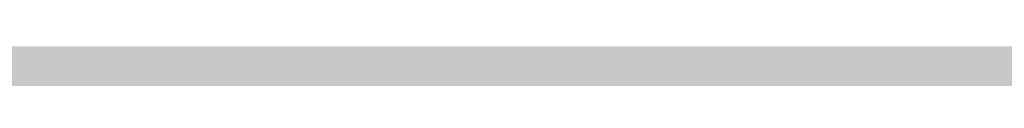
# Model space of a CAD drawing. Units: feet. Extents: x 3168 to 4724, y 827 to 1477.
# Tile 245 of 256: x 3383.8327 to 3384.3079, y 1099.0007 to 1099.0148. Entities that reach past the tile are written whole.
import ezdxf

# ---------------------------------------------------------------- set-up
doc = ezdxf.new("R2010")
doc.units = ezdxf.units.FT
doc.layers.add('A-ELEV', color=7, linetype='Continuous', lineweight=35)
doc.layers.add('A-ELEV-PATT', color=8, linetype='Continuous', lineweight=13)

msp = doc.modelspace()

# ---------------------------------------------------------------- hatches: boundary and pattern name
at = {"layer": 'A-ELEV-PATT'}
h = msp.add_hatch(color=256, dxfattribs=at)
h.dxf.hatch_style = 1
edge = h.paths.add_edge_path()
edge.add_ellipse((3552.90576, 979.22014), major_axis=(36.74492, 0), ratio=0.48484848, start_angle=0, end_angle=360)
edge = h.paths.add_edge_path()
edge.add_ellipse((3559.89164, 929.25228), major_axis=(36.74492, 0), ratio=0.48484848, start_angle=0, end_angle=360)
edge = h.paths.add_edge_path()
edge.add_line((3299.31681, 1198.60608), (3479.91671, 1198.60608))
edge.add_line((3479.91671, 1198.60608), (3479.91671, 1209.86857))
edge.add_spline(control_points=[(3479.91671, 1209.86857), (3464.30116, 1209.86857), (3448.6856, 1209.86857), (3410.94914, 1209.86857), (3388.82823, 1209.86857), (3355.64688, 1209.86857), (3344.58642, 1209.86857), (3327.99574, 1209.86857), (3322.46552, 1209.86857), (3314.17018, 1209.86857), (3311.40507, 1209.86857), (3307.2574, 1209.86857), (3305.87484, 1209.86857), (3303.801, 1209.86857), (3303.10973, 1209.86857), (3302.07281, 1209.86857), (3301.72717, 1209.86857), (3301.20871, 1209.86857), (3301.03589, 1209.86857), (3300.77666, 1209.86857), (3300.69025, 1209.86857), (3300.56064, 1209.86857), (3300.51743, 1209.86857), (3300.45263, 1209.86857), (3300.43102, 1209.86857), (3300.39862, 1209.86857), (3300.38782, 1209.86857), (3300.36622, 1209.86857), (3300.34568, 1209.86857), (3300.34555, 1209.86857), (3300.3455, 1209.86857), (3300.3433, 1209.86857), (3300.34115, 1209.86857), (3300.33791, 1209.86857), (3300.33683, 1209.86857), (3300.33394, 1209.86857), (3300.33213, 1209.86857), (3300.32552, 1209.86858), (3300.32071, 1209.86858), (3300.31092, 1209.86859), (3300.30595, 1209.8686), (3300.29051, 1209.86862), (3300.28005, 1209.86865), (3300.23243, 1209.86878), (3300.1953, 1209.86895), (3299.95107, 1209.87061), (3299.74482, 1209.87433), (3299.43683, 1209.88326), (3299.33439, 1209.88679), (3299.18108, 1209.89292), (3299.13003, 1209.8951), (3298.65222, 1209.9168), (3298.22946, 1209.94572), (3297.60163, 1210.00237), (3297.3934, 1210.02346), (3297.08265, 1210.05831), (3296.97933, 1210.07046), (3296.29295, 1210.15486), (3295.71815, 1210.24336), (3294.86872, 1210.39885), (3294.5877, 1210.45448), (3294.16934, 1210.54335), (3294.03042, 1210.57388), (3291.70715, 1211.1012), (3289.65359, 1211.81344), (3285.77626, 1213.56399), (3283.95141, 1214.60348), (3280.51216, 1216.98008), (3278.89724, 1218.31759), (3276.37991, 1220.82949), (3275.41604, 1221.91774), (3274.03934, 1223.7077), (3273.58104, 1224.34953), (3273.14323, 1225.01632)], knot_values=[39.119033, 39.119033, 39.119033, 39.119033, 39.286353, 39.286353, 39.523379, 39.523379, 39.641892, 39.641892, 39.701148, 39.701148, 39.730777, 39.730777, 39.745591, 39.745591, 39.752998, 39.752998, 39.756701, 39.756701, 39.758553, 39.758553, 39.759479, 39.759479, 39.759942, 39.759942, 39.760173, 39.760173, 39.760289, 39.760289, 39.760405, 39.760405, 39.760463, 39.760463, 39.763389, 39.763389, 39.764851, 39.764851, 39.767304, 39.767304, 39.773825, 39.773825, 39.78057, 39.78057, 39.79477, 39.79477, 39.845194, 39.845194, 40.126715, 40.126715, 40.267476, 40.267476, 40.337856, 40.337856, 40.927023, 40.927023, 41.221606, 41.221606, 41.368898, 41.368898, 42.202622, 42.202622, 42.619485, 42.619485, 42.827916, 42.827916, 46.118323, 46.118323, 49.408731, 49.408731, 52.699139, 52.699139, 54.927489, 54.927489, 56.104228, 56.104228, 56.104228, 56.104228], weights=[1, 1, 1, 1, 1, 1, 1, 1, 1, 1, 1, 1, 1, 1, 1, 1, 1, 1, 1, 1, 1, 1, 1, 1, 1, 1, 1, 1, 1, 1, 1, 1, 1, 1, 1, 1, 1, 1, 1, 1, 1, 1, 1, 1, 1, 1, 1, 1, 1, 1, 1, 1, 1, 1, 1, 1, 1, 1, 1, 1, 1, 1, 1, 1, 1, 1, 1, 1, 1, 1, 1, 1, 1, 1], degree=3, periodic=0)
edge.add_line((3273.14323, 1225.01632), (3273.14323, 1099.01632))
edge.add_line((3273.14323, 1099.01632), (3299.31681, 1099.01632))
edge.add_line((3299.31681, 1099.01632), (3299.31681, 1198.60608))
edge = h.paths.add_edge_path()
edge.add_line((3304.75844, 1324.15806), (3479.91671, 1324.15806))
edge.add_line((3479.91671, 1324.15806), (3479.91671, 1335.71462))
edge.add_line((3479.91671, 1335.71462), (3269.16163, 1335.71462))
edge.add_spline(control_points=[(3269.16163, 1335.71462), (3264.02423, 1335.71462), (3258.36412, 1328.95819), (3259.26431, 1323.90027)], knot_values=[0, 0, 0, 0, 15.412191, 15.412191, 15.412191, 15.412191], degree=3, periodic=0)
edge.add_line((3259.26431, 1323.90027), (3265.51685, 1288.76913))
edge.add_line((3265.51685, 1288.76913), (3275.2651, 1261.54563))
edge.add_line((3275.2651, 1261.54563), (3304.75844, 1261.54563))
edge.add_line((3304.75844, 1261.54563), (3304.75844, 1324.15806))
h = msp.add_hatch(color=256, dxfattribs=at)
h.dxf.hatch_style = 1
h.paths.add_polyline_path([(3384.52525, 1099.01632), (3335.02917, 1099.01632), (3299.31681, 1099.01632), (3273.14323, 1099.01632), (3217.56536, 1099.01632), (3168.06928, 827.11626), (3335.02917, 827.11626)])

# ---------------------------------------------------------------- linework, layer by layer
at = {"layer": 'A-ELEV'}
msp.add_open_spline([(3808.5202, 1099.01632), (3808.5202, 1141.41324), (3808.5202, 1183.81015), (3808.5202, 1226.63532), (3808.5202, 1227.06358), (3808.5202, 1227.49183), (3811.49187, 1248.99467), (3814.46354, 1270.49752), (3817.46523, 1292.21756), (3817.49525, 1292.43476), (3817.52526, 1292.65196), (3817.5728, 1310.10675), (3817.62034, 1327.56153), (3817.66788, 1345.01632), (3817.66788, 1345.45796), (3817.66788, 1345.89961), (3817.66788, 1346.45605), (3817.66788, 1346.57084), (3817.66788, 1346.75289), (3817.66788, 1346.82014), (3817.66788, 1346.93487), (3817.66788, 1346.98234), (3817.66788, 1347.03859), (3817.66788, 1347.04736), (3817.66788, 1347.07366), (3817.66788, 1347.0593), (3817.66788, 1347.06155), (3817.66788, 1347.06267), (3817.66788, 1347.06603), (3817.66787, 1347.06827), (3817.66787, 1347.075), (3817.66787, 1347.07949), (3817.66785, 1347.09294), (3817.66783, 1347.1019), (3817.66777, 1347.12879), (3817.6677, 1347.1467), (3817.66743, 1347.20042), (3817.66716, 1347.23619), (3817.6661, 1347.34338), (3817.66504, 1347.41469), (3817.66081, 1347.62809), (3817.65661, 1347.76971), (3817.63997, 1348.19249), (3817.62351, 1348.47159), (3817.55909, 1349.30007), (3817.49612, 1349.84059), (3817.25543, 1351.42416), (3817.02632, 1352.42879), (3816.30687, 1354.88891), (3815.74375, 1356.26873), (3814.46396, 1358.81921), (3813.74641, 1359.99097), (3812.19584, 1362.17234), (3811.36225, 1363.18212), (3809.58884, 1365.06901), (3808.64882, 1365.94611), (3806.65426, 1367.57962), (3805.5997, 1368.33615), (3803.35289, 1369.72233), (3802.16054, 1370.35239), (3799.60081, 1371.45359), (3798.23269, 1371.92548), (3795.28008, 1372.63462), (3793.69315, 1372.87207), (3791.86944, 1372.92648), (3791.74086, 1372.92922), (3791.35337, 1372.9341), (3791.09271, 1372.9329), (3790.30412, 1372.91507), (3789.76954, 1372.88419), (3789.20919, 1372.83024), (3789.19062, 1372.82842), (3789.13489, 1372.82291), (3789.0977, 1372.81914), (3789.04844, 1372.81401), (3789.0364, 1372.81274), (3789.00026, 1372.80892), (3788.97615, 1372.80633), (3788.9494, 1372.8034), (3788.94679, 1372.80312), (3788.94257, 1372.80266), (3788.94097, 1372.80248), (3788.93857, 1372.80222), (3788.93778, 1372.80213), (3788.93539, 1372.80187), (3788.86753, 1372.7944), (3788.75687, 1372.78223), (3788.70153, 1372.77614), (3788.53553, 1372.75788), (3788.42486, 1372.74571), (3788.09286, 1372.70918), (3787.87152, 1372.68484), (3787.20751, 1372.61179), (3786.76483, 1372.5631), (3785.43681, 1372.41701), (3784.55147, 1372.31962), (3781.89542, 1372.02744), (3780.12473, 1371.83266), (3774.81265, 1371.24831), (3771.27126, 1370.85874), (3760.64709, 1369.69004), (3753.56431, 1368.9109), (3732.31597, 1366.5735), (3718.15042, 1365.01523), (3694.00676, 1362.35933), (3684.02866, 1361.26169), (3674.05056, 1360.16406), (3664.60066, 1360.16406), (3655.15077, 1360.16406), (3626.80108, 1360.16406), (3607.90129, 1360.16406), (3551.20192, 1360.16406), (3513.40234, 1360.16406), (3467.72518, 1360.16406), (3459.8476, 1360.16406), (3436.21487, 1360.16406), (3420.45972, 1360.16406), (3373.19425, 1360.16406), (3341.68395, 1360.16406), (3302.84816, 1360.16406), (3295.52269, 1360.16406), (3286.03829, 1360.16406), (3283.87937, 1360.16406), (3277.40261, 1360.16406), (3273.08477, 1360.16406), (3267.73285, 1360.16406), (3266.69877, 1360.16406), (3263.59652, 1360.16406), (3261.52835, 1360.16406), (3259.23694, 1360.16406), (3259.0137, 1360.16406), (3258.34396, 1360.16406), (3257.89747, 1360.16406), (3257.431, 1360.16406), (3257.41102, 1360.16406), (3257.37057, 1360.16406), (3257.37547, 1360.16406), (3257.3746, 1360.16406), (3257.37394, 1360.16406), (3257.37196, 1360.16406), (3257.37064, 1360.16406), (3257.36667, 1360.16406), (3257.36403, 1360.16406), (3257.35611, 1360.16405), (3257.35083, 1360.16405), (3257.33499, 1360.16402), (3257.32443, 1360.164), (3257.29277, 1360.1639), (3257.27168, 1360.1638), (3257.20844, 1360.1634), (3257.16634, 1360.163), (3257.04021, 1360.16139), (3256.95635, 1360.15978), (3256.7055, 1360.15339), (3256.53924, 1360.14704), (3256.04357, 1360.12192), (3255.7173, 1360.0971), (3254.75245, 1360.00048), (3254.12797, 1359.90651), (3252.18007, 1359.52533), (3250.94157, 1359.14399), (3248.67018, 1358.24329), (3247.63574, 1357.72383), (3245.73263, 1356.60347), (3244.86339, 1356.00206), (3243.25311, 1354.74287), (3242.51197, 1354.08473), (3240.75105, 1352.34478), (3239.80096, 1351.22957), (3238.08777, 1348.87244), (3237.32469, 1347.63036), (3235.98251, 1344.97163), (3235.40221, 1343.55491), (3234.59108, 1340.81546), (3234.31088, 1339.54355), (3233.97649, 1336.80256), (3233.92211, 1335.33088), (3234.14892, 1332.59127), (3234.34953, 1331.3672), (3234.71989, 1329.99937), (3234.75242, 1329.88336), (3234.85362, 1329.5348), (3234.92589, 1329.30168), (3235.02484, 1329.00255), (3235.04692, 1328.93693), (3235.07764, 1328.84724), (3235.08592, 1328.8232), (3235.11094, 1328.75106), (3235.12783, 1328.70296), (3235.14799, 1328.64624), (3235.15106, 1328.63763), (3235.1561, 1328.62353), (3235.15806, 1328.61803), (3235.16021, 1328.61203), (3235.16561, 1328.59694), (3235.1801, 1328.55649), (3235.19026, 1328.5281), (3235.22076, 1328.44295), (3235.24108, 1328.38618), (3235.30207, 1328.21587), (3235.34273, 1328.10232), (3235.4647, 1327.7617), (3235.54601, 1327.53462), (3235.78995, 1326.85338), (3235.95258, 1326.39922), (3236.44046, 1325.03674), (3236.76571, 1324.12841), (3237.74148, 1321.40345), (3238.39198, 1319.5868), (3240.34351, 1314.13687), (3241.64452, 1310.50358), (3245.54757, 1299.60371), (3248.14961, 1292.33713), (3255.95571, 1270.53739), (3261.15977, 1256.00423), (3267.38762, 1238.612), (3268.4114, 1235.75294), (3269.51038, 1232.68386), (3269.58558, 1232.47385), (3269.70661, 1232.13585), (3269.75244, 1232.00786), (3269.82733, 1231.79873), (3269.85638, 1231.7176), (3269.90632, 1231.57812), (3269.92721, 1231.51978), (3269.97247, 1231.39341), (3269.99683, 1231.32537), (3270.0265, 1231.24251), (3270.03181, 1231.22768), (3270.04028, 1231.20402), (3270.03922, 1231.20698), (3270.03936, 1231.2066), (3270.03943, 1231.20641), (3270.03963, 1231.20585), (3270.03977, 1231.20547), (3270.04017, 1231.20433), (3270.04044, 1231.20358), (3270.04125, 1231.20131), (3270.0418, 1231.1998), (3270.04342, 1231.19527), (3270.0445, 1231.19225), (3270.04776, 1231.18318), (3270.04993, 1231.17714), (3270.05644, 1231.15903), (3270.06079, 1231.14696), (3270.07387, 1231.11076), (3270.08261, 1231.08666), (3270.10894, 1231.01441), (3270.1266, 1230.96635), (3270.17993, 1230.82246), (3270.21595, 1230.72692), (3270.32532, 1230.44151), (3270.40003, 1230.25281), (3270.62925, 1229.69144), (3270.78888, 1229.3235), (3271.28649, 1228.23832), (3271.6431, 1227.53975), (3272.77586, 1225.51528), (3273.61417, 1224.2605), (3275.41604, 1221.91774), (3276.37991, 1220.82949), (3278.89724, 1218.31759), (3280.51216, 1216.98008), (3283.95141, 1214.60348), (3285.77626, 1213.56399), (3289.65359, 1211.81344), (3291.70715, 1211.1012), (3294.03042, 1210.57388), (3294.16934, 1210.54335), (3294.5877, 1210.45448), (3294.86872, 1210.39885), (3295.71815, 1210.24336), (3296.29295, 1210.15486), (3296.97933, 1210.07046), (3297.08265, 1210.05831), (3297.3934, 1210.02346), (3297.60163, 1210.00237), (3298.22946, 1209.94572), (3298.65222, 1209.9168), (3299.13003, 1209.8951), (3299.18108, 1209.89292), (3299.33439, 1209.88679), (3299.43683, 1209.88326), (3299.74482, 1209.87433), (3299.95107, 1209.87061), (3300.1953, 1209.86895), (3300.23243, 1209.86878), (3300.28005, 1209.86865), (3300.29051, 1209.86862), (3300.30595, 1209.8686), (3300.31092, 1209.86859), (3300.32071, 1209.86858), (3300.32552, 1209.86858), (3300.33213, 1209.86857), (3300.33394, 1209.86857), (3300.33683, 1209.86857), (3300.33791, 1209.86857), (3300.34115, 1209.86857), (3300.3433, 1209.86857), (3300.3455, 1209.86857), (3300.34555, 1209.86857), (3300.34568, 1209.86857), (3300.36622, 1209.86857), (3300.38782, 1209.86857), (3300.39862, 1209.86857), (3300.43102, 1209.86857), (3300.45263, 1209.86857), (3300.51743, 1209.86857), (3300.56064, 1209.86857), (3300.69025, 1209.86857), (3300.77666, 1209.86857), (3301.03589, 1209.86857), (3301.20871, 1209.86857), (3301.72717, 1209.86857), (3302.07281, 1209.86857), (3303.10973, 1209.86857), (3303.801, 1209.86857), (3305.87484, 1209.86857), (3307.2574, 1209.86857), (3311.40507, 1209.86857), (3314.17018, 1209.86857), (3322.46552, 1209.86857), (3327.99574, 1209.86857), (3344.58642, 1209.86857), (3355.64688, 1209.86857), (3388.82823, 1209.86857), (3410.94914, 1209.86857), (3477.31185, 1209.86857), (3521.55366, 1209.86857), (3566.83618, 1209.86857), (3567.87689, 1209.86857), (3570.99902, 1209.86857), (3573.08043, 1209.86857), (3575.7814, 1209.86857), (3576.40094, 1209.86857), (3577.29582, 1209.86857), (3577.57115, 1209.86857), (3578.39715, 1209.86857), (3578.94781, 1209.86857), (3579.75649, 1209.86857), (3580.01451, 1209.86857), (3580.34274, 1209.86857), (3580.32686, 1209.86857), (3580.32717, 1209.86857), (3580.32732, 1209.86857), (3580.32778, 1209.86857), (3580.32809, 1209.86857), (3580.329, 1209.86857), (3580.32961, 1209.86857), (3580.33145, 1209.86857), (3580.33267, 1209.86857), (3580.33633, 1209.86857), (3580.33878, 1209.86857), (3580.34611, 1209.86856), (3580.35099, 1209.86856), (3580.36566, 1209.86854), (3580.37544, 1209.86852), (3580.4048, 1209.86845), (3580.42439, 1209.86838), (3580.48318, 1209.86808), (3580.52244, 1209.86779), (3580.64036, 1209.86662), (3580.71919, 1209.86545), (3580.95632, 1209.86077), (3581.11522, 1209.85607), (3581.59416, 1209.83723), (3581.91642, 1209.81833), (3582.88995, 1209.74243), (3583.54799, 1209.66617), (3585.53183, 1209.36062), (3586.86722, 1209.05389), (3589.47155, 1208.25247), (3590.74024, 1207.75785), (3591.99545, 1207.1588), (3592.05781, 1207.12874), (3592.24424, 1207.03795), (3592.36768, 1206.97663), (3592.73528, 1206.79036), (3592.97675, 1206.6631), (3593.24454, 1206.51644), (3593.27473, 1206.49982), (3593.36512, 1206.44984), (3593.42511, 1206.41633), (3593.60431, 1206.31529), (3593.72273, 1206.24721), (3593.85721, 1206.1684), (3593.87436, 1206.15832), (3593.92574, 1206.12804), (3593.9599, 1206.1078), (3594.06209, 1206.0469), (3594.12983, 1206.00607), (3594.20844, 1205.95817), (3594.21968, 1205.9513), (3594.25339, 1205.93069), (3594.27582, 1205.91692), (3594.34297, 1205.87554), (3594.38756, 1205.84785), (3594.43362, 1205.81905), (3594.43526, 1205.81802), (3594.44017, 1205.81495), (3594.44345, 1205.81289), (3594.44712, 1205.81059), (3594.44752, 1205.81035), (3594.44869, 1205.80961), (3594.44948, 1205.80912), (3594.45037, 1205.80856), (3594.45047, 1205.8085), (3594.4506, 1205.80842), (3594.4674, 1205.79789), (3594.49327, 1205.78167), (3594.5062, 1205.77357), (3594.54501, 1205.74925), (3594.57088, 1205.73303), (3594.64849, 1205.6844), (3594.70023, 1205.65197), (3594.85544, 1205.55469), (3594.95892, 1205.48984), (3595.26936, 1205.29528), (3595.47631, 1205.16558), (3596.09719, 1204.77646), (3596.5111, 1204.51705), (3597.75284, 1203.73883), (3598.58067, 1203.22001), (3601.06415, 1201.66355), (3602.71981, 1200.62591), (3607.68677, 1197.513), (3610.99809, 1195.43773), (3620.93202, 1189.2119), (3627.55464, 1185.06135), (3647.42251, 1172.60971), (3660.66775, 1164.30861), (3700.40348, 1139.40531), (3726.89397, 1122.80312), (3757.20572, 1103.80605), (3761.02697, 1101.41118), (3764.84822, 1099.01632), (3745.32827, 1099.01632), (3725.80832, 1099.01632), (3706.28837, 1099.01632), (3706.28837, 1108.45324), (3706.28837, 1117.89016), (3706.28837, 1127.32708), (3710.75075, 1127.32708), (3715.21314, 1127.32708), (3719.67553, 1127.32708)], degree=3, knots=[0, 0, 0, 0, 0.982037, 0.982037, 0.991957, 0.991957, 0.991957, 1.966522, 1.966522, 1.976367, 1.976367, 1.976367, 2.976367, 2.976367, 2.976367, 3.00169, 3.00169, 3.008272, 3.008272, 3.012129, 3.012129, 3.014851, 3.014851, 3.015353, 3.015353, 3.016359, 3.016359, 3.017365, 3.017365, 3.019376, 3.019376, 3.023398, 3.023398, 3.031442, 3.031442, 3.047531, 3.047531, 3.079708, 3.079708, 3.144063, 3.144063, 3.272772, 3.272772, 3.53019, 3.53019, 4.045026, 4.045026, 5.074698, 5.074698, 6.700878, 6.700878, 8.327058, 8.327058, 9.953238, 9.953238, 11.579418, 11.579418, 13.205598, 13.205598, 14.831778, 14.831778, 16.457958, 16.457958, 18.084138, 18.084138, 18.206872, 18.206872, 18.45234, 18.45234, 18.943275, 18.943275, 18.960093, 18.960093, 18.993729, 18.993729, 19.00461, 19.00461, 19.026374, 19.026374, 19.028737, 19.028737, 19.03018, 19.03018, 19.030897, 19.030897, 19.032332, 19.032332, 19.033766, 19.033766, 19.036636, 19.036636, 19.042374, 19.042374, 19.053851, 19.053851, 19.076805, 19.076805, 19.122714, 19.122714, 19.21453, 19.21453, 19.398163, 19.398163, 19.765429, 19.765429, 20.024128, 20.024128, 20.024128, 20.092031, 20.092031, 20.227836, 20.227836, 20.499446, 20.499446, 20.556051, 20.556051, 20.66926, 20.66926, 20.895678, 20.895678, 20.948316, 20.948316, 20.963829, 20.963829, 20.994855, 20.994855, 21.002285, 21.002285, 21.017146, 21.017146, 21.01875, 21.01875, 21.021959, 21.021959, 21.022102, 21.022102, 21.022249, 21.022249, 21.022708, 21.022708, 21.023627, 21.023627, 21.025464, 21.025464, 21.029138, 21.029138, 21.036486, 21.036486, 21.051183, 21.051183, 21.080575, 21.080575, 21.139361, 21.139361, 21.256932, 21.256932, 21.492073, 21.492073, 21.962356, 21.962356, 23.01002, 23.01002, 24.057684, 24.057684, 25.105348, 25.105348, 26.153011, 26.153011, 27.776787, 27.776787, 29.400562, 29.400562, 31.024337, 31.024337, 32.278801, 32.278801, 33.533265, 33.533265, 34.467568, 34.467568, 34.553971, 34.553971, 34.726776, 34.726776, 34.775309, 34.775309, 34.793079, 34.793079, 34.82862, 34.82862, 34.834979, 34.834979, 34.839039, 34.839039, 34.839411, 34.839411, 34.840285, 34.840285, 34.842034, 34.842034, 34.845531, 34.845531, 34.852525, 34.852525, 34.866512, 34.866512, 34.894488, 34.894488, 34.950439, 34.950439, 35.062342, 35.062342, 35.286147, 35.286147, 35.733758, 35.733758, 35.821815, 35.821815, 35.828283, 35.828283, 35.832225, 35.832225, 35.834724, 35.834724, 35.836521, 35.836521, 35.838617, 35.838617, 35.839073, 35.839073, 35.839345, 35.839345, 35.839617, 35.839617, 35.840161, 35.840161, 35.841249, 35.841249, 35.843425, 35.843425, 35.847778, 35.847778, 35.856482, 35.856482, 35.873891, 35.873891, 35.908709, 35.908709, 35.978345, 35.978345, 36.117617, 36.117617, 36.396161, 36.396161, 36.953248, 36.953248, 38.067423, 38.067423, 40.295772, 40.295772, 42.524122, 42.524122, 45.81453, 45.81453, 49.104937, 49.104937, 52.395345, 52.395345, 52.603776, 52.603776, 53.020639, 53.020639, 53.854363, 53.854363, 54.001655, 54.001655, 54.296238, 54.296238, 54.885405, 54.885405, 54.955785, 54.955785, 55.096546, 55.096546, 55.378067, 55.378067, 55.42849, 55.42849, 55.442691, 55.442691, 55.449436, 55.449436, 55.455957, 55.455957, 55.458409, 55.458409, 55.459872, 55.459872, 55.462798, 55.462798, 55.462856, 55.462856, 55.462972, 55.462972, 55.463088, 55.463088, 55.463319, 55.463319, 55.463782, 55.463782, 55.464708, 55.464708, 55.46656, 55.46656, 55.470263, 55.470263, 55.47767, 55.47767, 55.492484, 55.492484, 55.522112, 55.522112, 55.581369, 55.581369, 55.699882, 55.699882, 55.936907, 55.936907, 56.410959, 56.410959, 56.42211, 56.42211, 56.444413, 56.444413, 56.451051, 56.451051, 56.454001, 56.454001, 56.459901, 56.459901, 56.462666, 56.462666, 56.463418, 56.463418, 56.464171, 56.464171, 56.465675, 56.465675, 56.468684, 56.468684, 56.474702, 56.474702, 56.486738, 56.486738, 56.51081, 56.51081, 56.558955, 56.558955, 56.655243, 56.655243, 56.847821, 56.847821, 57.232975, 57.232975, 58.003284, 58.003284, 59.543901, 59.543901, 62.625137, 62.625137, 68.787607, 68.787607, 74.950078, 74.950078, 75.27336, 75.27336, 75.919923, 75.919923, 77.213051, 77.213051, 77.377769, 77.377769, 77.707206, 77.707206, 78.366079, 78.366079, 78.462532, 78.462532, 78.655436, 78.655436, 79.041245, 79.041245, 79.105735, 79.105735, 79.234714, 79.234714, 79.492672, 79.492672, 79.502197, 79.502197, 79.521249, 79.521249, 79.523534, 79.523534, 79.528103, 79.528103, 79.528682, 79.528682, 79.528885, 79.528885, 79.529089, 79.529089, 79.529495, 79.529495, 79.530308, 79.530308, 79.531935, 79.531935, 79.535187, 79.535187, 79.541693, 79.541693, 79.554704, 79.554704, 79.580725, 79.580725, 79.632769, 79.632769, 79.736856, 79.736856, 79.94503, 79.94503, 80.361377, 80.361377, 80.421435, 80.421435, 80.421435, 81.421435, 81.421435, 81.421435, 82.421435, 82.421435, 82.421435, 83.421435, 83.421435, 83.421435, 83.421435], dxfattribs=at)

doc.saveas('drawing.dxf')
